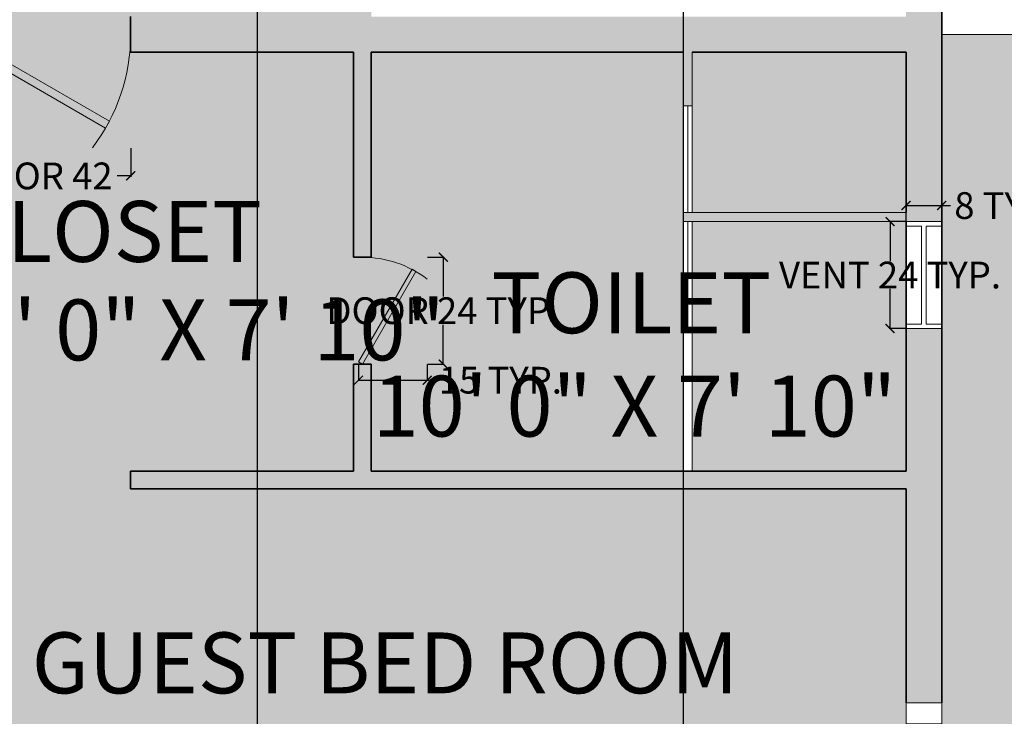
# Model space of a CAD drawing. Units: inches. Extents: x 1704 to 6393, y -157 to 1172.
# Tile 37 of 122: x 2398 to 2619, y 215 to 372. Entities that reach past the tile are written whole.
import ezdxf

# ---------------------------------------------------------------- set-up
doc = ezdxf.new("R2010")
doc.units = ezdxf.units.IN
doc.header["$MEASUREMENT"] = 0
for name, color, linetype, lineweight in [('A-ANNO-DIMS', 7, 'Continuous', 13), ('A-AREA-IDEN', 7, 'Continuous', 18), ('A-WALL-PATT', 7, 'Continuous', 13), ('DOORS', 160, 'Continuous', 18), ('GLASS PANEL FASADE', 4, 'Continuous', 18), ('L-HRDS', 8, 'Continuous', 18), ('L-PVMT-PATT', 8, 'Continuous', 13), ('WALLS', 7, 'Continuous', 35), ('WINDOWS', 2, 'Continuous', 18)]:
    doc.layers.add(name, color=color, linetype=linetype, lineweight=lineweight)
doc.layers.add('A-FLOR-PATT', color=7, linetype='Continuous', lineweight=13, true_color=0xf2f2f2)
doc.layers.add('L-HRDS-PATT', color=9, linetype='Continuous', lineweight=13, true_color=0xc5c1ba)
doc.styles.get("Standard").update_dxf_attribs({"font": 'arial.ttf'})
doc.dimstyles.get("Standard").update_dxf_attribs({"dimtxt": 6, "dimasz": 2, "dimexe": 0.18, "dimexo": 0.0625, "dimgap": 0.09, "dimtad": 0, "dimtih": 1, "dimtoh": 1, "dimdec": 1, "dimzin": 0, "dimdsep": 46, "dimlunit": 3, "dimtxsty": 'Standard', "dimblk": 'ARCHTICK', "dimcen": 0.09, "dimadec": 0, "dimazin": 0, "dimtfac": 1, "dimtdec": 1, "dimtofl": 0, "dimtmove": 0, "dimatfit": 3, "dimfxl": 1, "dimtolj": 1, "dimtzin": 0, "dimarcsym": 0})

# ---------------------------------------------------------------- blocks, each defined once
blk = doc.blocks.new('Door - Left Hung 36 in.')
blk.add_lwpolyline([(0.75, -1.3), (0, 0), (31.18, 18), (31.93, 16.7)], close=True)
blk.add_arc((0, 0), 36, 0, 37.3101)
blk = doc.blocks.new('WIN-SLIDER-72')
for p, q in [((0, 72), (0, 0)), ((0, 72), (8, 72)), ((8, 66.25), (8, 72)), ((0, 67.23), (8, 67.23)), ((1.17, 36), (1.17, 64.3)), ((8, 7.7), (8, 64.3)), ((3.12, 37.95), (3.12, 62.35)), ((4.1, 37.95), (4.1, 62.35)), ((5.07, 37.95), (5.07, 62.35)), ((2.14, 37.95), (2.14, 42.14)), ((5.07, 36), (5.07, 7.7)), ((1.17, 9.65), (1.17, 34.05)), ((2.14, 9.65), (2.14, 34.05)), ((3.12, 9.65), (3.12, 34.05)), ((4.1, 34.05), (4.1, 29.86)), ((0, 4.77), (8, 4.77)), ((8, 5.75), (8, 0)), ((0, 0), (8, 0))]:
    blk.add_line(p, q)
for points in [[(8, 64.3), (8, 66.25), (0, 66.25), (0, 64.3)], [(5.07, 62.35), (5.07, 64.3), (3.12, 64.3), (3.12, 62.35)], [(2.14, 42.65), (1.85, 42.14), (2.44, 42.14)], [(5.07, 36), (5.07, 37.95), (3.12, 37.95), (3.12, 36)], [(3.12, 34.05), (3.12, 36), (1.17, 36), (1.17, 34.05)], [(4.1, 29.35), (3.8, 29.86), (4.39, 29.86)], [(3.12, 7.7), (3.12, 9.65), (1.17, 9.65), (1.17, 7.7)], [(8, 7.7), (8, 5.75), (0, 5.75), (0, 7.7)]]:
    blk.add_lwpolyline(points, close=True)
blk = doc.blocks.new('WIN-VENT-24')
for p, q in [((0, 0), (0, 24)), ((0, 24), (8, 24)), ((0, 23), (3.5, 23)), ((3.5, 23), (3.5, 1)), ((4.5, 23), (8, 23)), ((4.5, 23), (4.5, 1)), ((8, 24), (8, 0)), ((3.5, 1), (0, 1)), ((8, 1), (4.5, 1)), ((8, 0), (0, 0))]:
    blk.add_line(p, q)
blk = doc.blocks.new('_ArchTick')
at = {"color": 0, "linetype": 'ByBlock', "const_width": 0.15}
blk.add_lwpolyline([(-0.5, -0.5), (0.5, 0.5)], dxfattribs=at)
blk = doc.blocks.new('*D30')
at = {"layer": 'A-ANNO-DIMS', "color": 0, "lineweight": -2, "transparency": 16777216}
for p, q in [((2381.35, 342.69), (2381.35, 336.28)), ((2423.35, 342.69), (2423.35, 336.28)), ((2381.35, 336.46), (2384.4, 336.46)), ((2423.35, 336.46), (2420.29, 336.46))]:
    blk.add_line(p, q, dxfattribs=at)
at = {"layer": 'Defpoints', "color": 0, "lineweight": -3, "transparency": 16777216}
for p in [(2381.35, 342.76), (2423.35, 342.76), (2423.35, 336.46)]:
    blk.add_point(p, dxfattribs=at)
at = {"layer": 'A-ANNO-DIMS', "color": 0, "lineweight": -2, "transparency": 16777216, "xscale": 2, "yscale": 2, "zscale": 2, "rotation": 180}
blk.add_blockref('_ArchTick', (2381.35, 336.46), dxfattribs=at)
at = {"layer": 'A-ANNO-DIMS', "color": 0, "lineweight": -2, "transparency": 16777216, "xscale": 2, "yscale": 2, "zscale": 2}
blk.add_blockref('_ArchTick', (2423.35, 336.46), dxfattribs=at)
at = {"layer": 'A-ANNO-DIMS', "color": 0, "transparency": 16777216, "insert": (2402.35, 336.46), "char_height": 6, "attachment_point": 5}
blk.add_mtext('\\A1;DOOR 42', dxfattribs=at)
blk = doc.blocks.new('*D32')
at = {"layer": 'A-ANNO-DIMS', "color": 0, "lineweight": -2, "transparency": 16777216}
for p, q in [((2489.96, 318.21), (2493.68, 318.21)), ((2493.5, 318.21), (2493.5, 309.41)), ((2493.5, 294.21), (2493.5, 303.02)), ((2489.96, 294.21), (2493.68, 294.21))]:
    blk.add_line(p, q, dxfattribs=at)
at = {"layer": 'Defpoints', "color": 0, "lineweight": -3, "transparency": 16777216}
for p in [(2489.9, 318.21), (2493.5, 318.21), (2489.9, 294.21)]:
    blk.add_point(p, dxfattribs=at)
at = {"layer": 'A-ANNO-DIMS', "color": 0, "lineweight": -2, "transparency": 16777216, "xscale": 2, "yscale": 2, "zscale": 2}
for p, rotation in [((2493.5, 318.21), 90), ((2493.5, 294.21), 270)]:
    blk.add_blockref('_ArchTick', p, dxfattribs=dict(at, rotation=rotation))
at = {"layer": 'A-ANNO-DIMS', "color": 0, "transparency": 16777216, "insert": (2493.5, 306.21), "char_height": 6, "attachment_point": 5}
blk.add_mtext('\\A1;DOOR 24 TYP.', dxfattribs=at)
blk = doc.blocks.new('*D33')
at = {"layer": 'A-ANNO-DIMS', "color": 0, "lineweight": -2, "transparency": 16777216}
for p, q in [((2474.48, 294.15), (2474.48, 290.43)), ((2489.9, 294.15), (2489.9, 290.43)), ((2474.48, 290.61), (2489.9, 290.61)), ((2489.9, 290.61), (2491.9, 290.61))]:
    blk.add_line(p, q, dxfattribs=at)
at = {"layer": 'Defpoints', "color": 0, "lineweight": -3, "transparency": 16777216}
for p in [(2474.48, 294.21), (2489.9, 294.21), (2489.9, 290.61)]:
    blk.add_point(p, dxfattribs=at)
at = {"layer": 'A-ANNO-DIMS', "color": 0, "lineweight": -2, "transparency": 16777216, "xscale": 2, "yscale": 2, "zscale": 2, "rotation": 180}
blk.add_blockref('_ArchTick', (2474.48, 290.61), dxfattribs=at)
at = {"layer": 'A-ANNO-DIMS', "color": 0, "lineweight": -2, "transparency": 16777216, "xscale": 2, "yscale": 2, "zscale": 2}
blk.add_blockref('_ArchTick', (2489.9, 290.61), dxfattribs=at)
at = {"layer": 'A-ANNO-DIMS', "color": 0, "transparency": 16777216, "insert": (2506.31, 290.61), "char_height": 6, "attachment_point": 5}
blk.add_mtext('\\A1;15 TYP.', dxfattribs=at)
blk = doc.blocks.new('*D42')
at = {"layer": 'A-ANNO-DIMS', "color": 0, "lineweight": -2, "transparency": 16777216}
for p, q in [((2597.29, 326.21), (2593.57, 326.21)), ((2593.75, 326.21), (2593.75, 317.32)), ((2593.75, 302.21), (2593.75, 311.11)), ((2597.29, 302.21), (2593.57, 302.21))]:
    blk.add_line(p, q, dxfattribs=at)
at = {"layer": 'Defpoints', "color": 0, "lineweight": -3, "transparency": 16777216}
for p in [(2593.75, 326.21), (2597.35, 326.21), (2597.35, 302.21)]:
    blk.add_point(p, dxfattribs=at)
at = {"layer": 'A-ANNO-DIMS', "color": 0, "lineweight": -2, "transparency": 16777216, "xscale": 2, "yscale": 2, "zscale": 2}
for p, rotation in [((2593.75, 326.21), 90), ((2593.75, 302.21), 270)]:
    blk.add_blockref('_ArchTick', p, dxfattribs=dict(at, rotation=rotation))
at = {"layer": 'A-ANNO-DIMS', "color": 0, "transparency": 16777216, "insert": (2593.75, 314.21), "char_height": 6, "attachment_point": 5}
blk.add_mtext('\\A1;VENT 24 TYP.', dxfattribs=at)
blk = doc.blocks.new('*D43')
at = {"layer": 'A-ANNO-DIMS', "color": 0, "lineweight": -2, "transparency": 16777216}
for p, q in [((2597.35, 326.28), (2597.35, 329.99)), ((2597.35, 329.81), (2605.35, 329.81)), ((2605.35, 326.28), (2605.35, 329.99)), ((2605.35, 329.81), (2607.35, 329.81))]:
    blk.add_line(p, q, dxfattribs=at)
at = {"layer": 'Defpoints', "color": 0, "lineweight": -3, "transparency": 16777216}
for p in [(2605.35, 329.81), (2597.35, 326.21), (2605.35, 326.21)]:
    blk.add_point(p, dxfattribs=at)
at = {"layer": 'A-ANNO-DIMS', "color": 0, "lineweight": -2, "transparency": 16777216, "xscale": 2, "yscale": 2, "zscale": 2, "rotation": 180}
blk.add_blockref('_ArchTick', (2597.35, 329.81), dxfattribs=at)
at = {"layer": 'A-ANNO-DIMS', "color": 0, "lineweight": -2, "transparency": 16777216, "xscale": 2, "yscale": 2, "zscale": 2}
blk.add_blockref('_ArchTick', (2605.35, 329.81), dxfattribs=at)
at = {"layer": 'A-ANNO-DIMS', "color": 0, "transparency": 16777216, "insert": (2619.71, 329.81), "char_height": 6, "attachment_point": 5}
blk.add_mtext('\\A1;8 TYP.', dxfattribs=at)
blk = doc.blocks.new('*D93')
at = {"layer": 'A-ANNO-DIMS', "color": 0, "lineweight": -2, "transparency": 16777216}
for p, q in [((2605.29, 895.21), (1829.7, 895.21)), ((1829.88, 895.21), (1829.88, 495.87)), ((1829.88, 90.21), (1829.88, 489.56)), ((2605.29, 90.21), (1829.7, 90.21))]:
    blk.add_line(p, q, dxfattribs=at)
at = {"layer": 'Defpoints', "color": 0, "lineweight": -3, "transparency": 16777216}
for p in [(2605.35, 895.21), (1829.88, 90.21), (2605.35, 90.21)]:
    blk.add_point(p, dxfattribs=at)
at = {"layer": 'A-ANNO-DIMS', "color": 0, "lineweight": -2, "transparency": 16777216, "xscale": 2, "yscale": 2, "zscale": 2}
for p, rotation in [((1829.88, 895.21), 90), ((1829.88, 90.21), 270)]:
    blk.add_blockref('_ArchTick', p, dxfattribs=dict(at, rotation=rotation))
at = {"layer": 'A-ANNO-DIMS', "color": 0, "transparency": 16777216, "insert": (1829.88, 492.71), "char_height": 6, "attachment_point": 5}
blk.add_mtext('\\A1;805', dxfattribs=at)
blk = doc.blocks.new('*D105')
at = {"layer": 'A-ANNO-DIMS', "color": 0, "lineweight": -2, "transparency": 16777216}
for p, q in [((2451.74, 615.15), (2451.74, -64.97)), ((2547.35, 615.15), (2547.35, -64.97)), ((2451.74, -64.79), (2489.91, -64.79)), ((2547.35, -64.79), (2509.18, -64.79))]:
    blk.add_line(p, q, dxfattribs=at)
at = {"layer": 'Defpoints', "color": 0, "lineweight": -3, "transparency": 16777216}
for p in [(2451.74, 615.21), (2547.35, 615.21), (2547.35, -64.79)]:
    blk.add_point(p, dxfattribs=at)
at = {"layer": 'A-ANNO-DIMS', "color": 0, "lineweight": -2, "transparency": 16777216, "xscale": 2, "yscale": 2, "zscale": 2, "rotation": 180}
blk.add_blockref('_ArchTick', (2451.74, -64.79), dxfattribs=at)
at = {"layer": 'A-ANNO-DIMS', "color": 0, "lineweight": -2, "transparency": 16777216, "xscale": 2, "yscale": 2, "zscale": 2}
blk.add_blockref('_ArchTick', (2547.35, -64.79), dxfattribs=at)
at = {"layer": 'A-ANNO-DIMS', "color": 0, "transparency": 16777216, "insert": (2499.54, -64.79), "char_height": 6, "attachment_point": 5}
blk.add_mtext('\\A1;95.61', dxfattribs=at)

msp = doc.modelspace()

# ---------------------------------------------------------------- hatches: boundary and pattern name
at = {"layer": 'A-FLOR-PATT', "transparency": 33554528}
h = msp.add_hatch(color=256, dxfattribs=at)
h.dxf.hatch_style = 1
h.paths.add_polyline_path([(2325.349, 863.213), (2325.349, 887.213), (2263.349, 887.213), (2167.349, 887.213), (2081.349, 887.213), (2081.349, 719.213), (2277.349, 719.213), (2277.349, 711.213), (2277.349, 372.213), (2349.349, 372.213), (2381.349, 372.213), (2381.349, 364.213), (2353.349, 364.213), (2353.349, 270.213), (2381.349, 270.213), (2381.349, 266.213), (2357.349, 266.213), (2357.349, 98.213), (2381.349, 98.213), (2385.181, 98.213), (2386.482, 98.213), (2424.215, 98.213), (2425.516, 98.213), (2429.349, 98.213), (2597.349, 98.213), (2597.349, 146.213), (2597.349, 218.213), (2597.349, 266.213), (2423.349, 266.213), (2423.349, 270.213), (2473.349, 270.213), (2473.349, 294.213), (2477.349, 294.213), (2477.349, 270.213), (2547.349, 270.213), (2547.349, 364.213), (2477.349, 364.213), (2477.349, 318.213), (2473.349, 318.213), (2473.349, 364.213), (2423.349, 364.213), (2423.349, 372.213), (2469.349, 372.213), (2469.349, 459.213), (2469.349, 538.213), (2350.349, 538.213), (2350.349, 565.713), (2358.349, 565.713), (2358.349, 545.213), (2420.349, 545.213), (2420.349, 610.213), (2358.349, 610.213), (2358.349, 589.713), (2350.349, 589.713), (2350.349, 615.213), (2425.349, 615.213), (2425.349, 607.213), (2425.349, 546.213), (2469.349, 546.213), (2514.349, 546.213), (2514.349, 607.213), (2449.349, 607.213), (2449.349, 615.213), (2451.738, 615.213), (2451.738, 659.213), (2427.738, 659.213), (2427.738, 665.213), (2367.738, 665.213), (2367.738, 667.213), (2367.738, 711.213), (2325.349, 711.213), (2325.349, 719.213), (2325.349, 755.213), (2325.349, 763.213)])
h.paths.add_polyline_path([(2233.858, 822.533, -0.187247), (2233.858, 809.14), (2231.697, 808.804, 0.0848928), (2233.131, 814.486), (2230.424, 814.486, -0.1042581), (2228.553, 808.313), (2217.751, 807.156, -0.2222222), (2217.751, 824.517), (2228.553, 823.359, -0.1042581), (2230.424, 817.186), (2233.131, 817.186, 0.0848928), (2231.697, 822.868)], flags=16)
h.paths.add_polyline_path([(2213.621, 833.197), (2213.621, 798.475), (2156.048, 798.475), (2156.048, 833.197)], flags=16)
h.paths.add_polyline_path([(2203.932, 848.099), (2205.089, 837.296, -0.2222222), (2187.728, 837.296), (2188.885, 848.099, -0.1042581), (2195.058, 849.969), (2195.058, 852.676, 0.0848928), (2189.377, 851.242), (2189.712, 853.404, -0.187247), (2203.105, 853.404), (2203.44, 851.242, 0.0848928), (2197.759, 852.676), (2197.759, 849.969, -0.1042581)], flags=16)
h.paths.add_polyline_path([(2181.941, 837.296, -0.2222222), (2164.58, 837.296), (2165.737, 848.099, -0.1042581), (2171.91, 849.969), (2171.91, 852.676, 0.0848928), (2166.229, 851.242), (2166.564, 853.404, -0.187247), (2179.957, 853.404), (2180.292, 851.242, 0.0848928), (2174.611, 852.676), (2174.611, 849.969, -0.1042581), (2180.784, 848.099)], flags=16)
h.paths.add_polyline_path([(2205.089, 794.376), (2203.932, 783.574, -0.1042581), (2197.759, 781.703), (2197.759, 778.996, 0.0848928), (2203.44, 780.43), (2203.105, 778.269, -0.187247), (2189.712, 778.269), (2189.377, 780.43, 0.0848928), (2195.058, 778.996), (2195.058, 781.703, -0.1042581), (2188.885, 783.574), (2187.728, 794.376, -0.2222222)], flags=16)
h.paths.add_polyline_path([(2181.941, 794.376), (2180.784, 783.574, -0.1042581), (2174.611, 781.703), (2174.611, 778.996, 0.0848928), (2180.292, 780.43), (2179.957, 778.269, -0.187247), (2166.564, 778.269), (2166.229, 780.43, 0.0848928), (2171.91, 778.996), (2171.91, 781.703, -0.1042581), (2165.737, 783.574), (2164.58, 794.376, -0.2222222)], flags=16)
h.paths.add_polyline_path([(2151.918, 807.156), (2141.116, 808.313, -0.1042581), (2139.245, 814.486), (2136.539, 814.486, 0.0848928), (2137.972, 808.804), (2135.811, 809.14, -0.187247), (2135.811, 822.533), (2137.972, 822.868, 0.0848928), (2136.539, 817.186), (2139.245, 817.186, -0.1042581), (2141.116, 823.359), (2151.918, 824.517, -0.2222222)], flags=16)
h.paths.add_polyline_path([(2357.868, 363.41), (2358.814, 363.41, 0.7537605)], flags=16)
h.paths.add_polyline_path([(2372.241, 363.117), (2372.248, 363.117), (2372.248, 363.343), (2371.302, 363.343), (2371.302, 363.139, -1.3603913)], flags=16)
h.paths.add_polyline_path([(2371.309, 272.716), (2371.302, 272.716), (2371.302, 272.49), (2372.248, 272.49), (2372.248, 272.693, -1.3603913)], flags=16)
h.paths.add_polyline_path([(2357.875, 272.716), (2357.868, 272.716), (2357.868, 272.49), (2358.814, 272.49), (2358.814, 272.693, -1.3603913)], flags=16)
h.paths.add_polyline_path([(2353.769, 363.074), (2376.347, 363.074), (2376.347, 272.759), (2353.769, 272.759)], flags=16)
h.paths.add_polyline_path([(2354.772, 362.07), (2375.344, 362.07), (2375.344, 273.762), (2354.772, 273.762)], flags=0)
h.paths.add_polyline_path([(2357.868, 363.343), (2358.814, 363.343), (2358.814, 363.117), (2357.868, 363.117)], flags=16)
h.paths.add_polyline_path([(2359.288, 359.184), (2359.288, 360.063), (2370.828, 360.063), (2370.828, 359.184), (2374.332, 359.184), (2374.332, 358.464), (2372.835, 358.464), (2372.835, 357.541), (2374.332, 357.541), (2374.332, 356.82), (2372.835, 356.82), (2372.835, 355.898), (2374.332, 355.898), (2374.332, 355.177), (2372.835, 355.177), (2372.835, 354.254), (2374.332, 354.254), (2374.332, 353.534), (2372.835, 353.534), (2372.835, 352.611), (2374.332, 352.611), (2374.332, 351.89), (2372.835, 351.89), (2372.835, 350.968), (2374.332, 350.968), (2374.332, 350.247), (2372.835, 350.247), (2372.835, 349.324), (2374.332, 349.324), (2374.332, 348.604), (2372.835, 348.604), (2372.835, 347.681), (2374.332, 347.681), (2374.332, 346.96), (2372.835, 346.96), (2372.835, 346.038), (2374.332, 346.038), (2374.332, 345.317), (2372.835, 345.317), (2372.835, 344.395), (2374.332, 344.395), (2374.332, 343.674), (2372.835, 343.674), (2372.835, 342.751), (2374.332, 342.751), (2374.332, 342.03), (2372.835, 342.03), (2372.835, 341.108), (2374.332, 341.108), (2374.332, 340.387), (2372.835, 340.387), (2372.835, 339.465), (2374.332, 339.465), (2374.332, 338.744), (2372.835, 338.744), (2372.835, 337.821), (2374.332, 337.821), (2374.332, 337.1), (2372.835, 337.1), (2372.835, 336.178), (2374.332, 336.178), (2374.332, 335.457), (2372.835, 335.457), (2372.835, 334.535), (2374.332, 334.535), (2374.332, 333.814), (2372.835, 333.814), (2372.835, 332.891), (2374.332, 332.891), (2374.332, 332.171), (2372.835, 332.171), (2372.835, 331.248), (2374.332, 331.248), (2374.332, 330.527), (2372.835, 330.527), (2372.835, 329.605), (2374.332, 329.605), (2374.332, 328.884), (2372.835, 328.884), (2372.835, 327.961), (2374.332, 327.961), (2374.332, 327.241), (2372.835, 327.241), (2372.835, 326.318), (2374.332, 326.318), (2374.332, 325.597), (2372.835, 325.597), (2372.835, 324.675), (2374.332, 324.675), (2374.332, 323.954), (2372.835, 323.954), (2372.835, 323.031), (2374.332, 323.031), (2374.332, 322.311), (2372.835, 322.311), (2372.835, 321.388), (2374.332, 321.388), (2374.332, 320.667), (2372.835, 320.667), (2372.835, 319.745), (2374.332, 319.745), (2374.332, 319.024), (2372.835, 319.024), (2372.835, 318.102), (2374.332, 318.102), (2374.332, 317.381), (2372.835, 317.381), (2372.835, 316.458), (2374.332, 316.458), (2374.332, 315.737), (2372.835, 315.737), (2372.835, 314.815), (2374.332, 314.815), (2374.332, 314.094), (2372.835, 314.094), (2372.835, 313.172), (2374.332, 313.172), (2374.332, 312.451), (2372.835, 312.451), (2372.835, 311.528), (2374.332, 311.528), (2374.332, 310.807), (2372.835, 310.807), (2372.835, 309.885), (2374.332, 309.885), (2374.332, 309.164), (2372.835, 309.164), (2372.835, 308.242), (2374.332, 308.242), (2374.332, 307.521), (2372.835, 307.521), (2372.835, 306.598), (2374.332, 306.598), (2374.332, 305.878), (2372.835, 305.878), (2372.835, 304.955), (2374.332, 304.955), (2374.332, 304.234), (2372.835, 304.234), (2372.835, 303.312), (2374.332, 303.312), (2374.332, 302.591), (2372.835, 302.591), (2372.835, 301.668), (2374.332, 301.668), (2374.332, 300.948), (2372.835, 300.948), (2372.835, 300.025), (2374.332, 300.025), (2374.332, 299.304), (2372.835, 299.304), (2372.835, 298.382), (2374.332, 298.382), (2374.332, 297.661), (2372.835, 297.661), (2372.835, 296.738), (2374.332, 296.738), (2374.332, 296.018), (2372.835, 296.018), (2372.835, 295.095), (2374.332, 295.095), (2374.332, 294.374), (2372.835, 294.374), (2372.835, 293.452), (2374.332, 293.452), (2374.332, 292.731), (2372.835, 292.731), (2372.835, 291.809), (2374.332, 291.809), (2374.332, 291.088), (2372.835, 291.088), (2372.835, 290.165), (2374.332, 290.165), (2374.332, 289.444), (2372.835, 289.444), (2372.835, 288.522), (2374.332, 288.522), (2374.332, 287.801), (2372.835, 287.801), (2372.835, 286.879), (2374.332, 286.879), (2374.332, 286.158), (2372.835, 286.158), (2372.835, 285.235), (2374.332, 285.235), (2374.332, 284.514), (2372.835, 284.514), (2372.835, 283.592), (2374.332, 283.592), (2374.332, 282.871), (2372.835, 282.871), (2372.835, 281.949), (2374.332, 281.949), (2374.332, 281.228), (2372.835, 281.228), (2372.835, 280.305), (2374.332, 280.305), (2374.332, 279.585), (2372.835, 279.585), (2372.835, 278.662), (2374.332, 278.662), (2374.332, 277.941), (2372.835, 277.941), (2372.835, 277.019), (2374.332, 277.019), (2374.332, 276.298), (2370.828, 276.298), (2370.828, 275.769), (2359.288, 275.769), (2359.288, 276.298), (2355.784, 276.298), (2355.784, 277.019), (2357.281, 277.019), (2357.281, 277.941), (2355.784, 277.941), (2355.784, 278.662), (2357.281, 278.662), (2357.281, 279.585), (2355.784, 279.585), (2355.784, 280.305), (2357.281, 280.305), (2357.281, 281.228), (2355.784, 281.228), (2355.784, 281.949), (2357.281, 281.949), (2357.281, 282.871), (2355.784, 282.871), (2355.784, 283.592), (2357.281, 283.592), (2357.281, 284.514), (2355.784, 284.514), (2355.784, 285.235), (2357.281, 285.235), (2357.281, 286.158), (2355.784, 286.158), (2355.784, 286.879), (2357.281, 286.879), (2357.281, 287.801), (2355.784, 287.801), (2355.784, 288.522), (2357.281, 288.522), (2357.281, 289.444), (2355.784, 289.444), (2355.784, 290.165), (2357.281, 290.165), (2357.281, 291.088), (2355.784, 291.088), (2355.784, 291.809), (2357.281, 291.809), (2357.281, 292.731), (2355.784, 292.731), (2355.784, 293.452), (2357.281, 293.452), (2357.281, 294.374), (2355.784, 294.374), (2355.784, 295.095), (2357.281, 295.095), (2357.281, 296.018), (2355.784, 296.018), (2355.784, 296.738), (2357.281, 296.738), (2357.281, 297.661), (2355.784, 297.661), (2355.784, 298.382), (2357.281, 298.382), (2357.281, 299.304), (2355.784, 299.304), (2355.784, 300.025), (2357.281, 300.025), (2357.281, 300.948), (2355.784, 300.948), (2355.784, 301.668), (2357.281, 301.668), (2357.281, 302.591), (2355.784, 302.591), (2355.784, 303.312), (2357.281, 303.312), (2357.281, 304.234), (2355.784, 304.234), (2355.784, 304.955), (2357.281, 304.955), (2357.281, 305.878), (2355.784, 305.878), (2355.784, 306.598), (2357.281, 306.598), (2357.281, 307.521), (2355.784, 307.521), (2355.784, 308.242), (2357.281, 308.242), (2357.281, 309.164), (2355.784, 309.164), (2355.784, 309.885), (2357.281, 309.885), (2357.281, 310.807), (2355.784, 310.807), (2355.784, 311.528), (2357.281, 311.528), (2357.281, 312.451), (2355.784, 312.451), (2355.784, 313.172), (2357.281, 313.172), (2357.281, 314.094), (2355.784, 314.094), (2355.784, 314.815), (2357.281, 314.815), (2357.281, 315.737), (2355.784, 315.737), (2355.784, 316.458), (2357.281, 316.458), (2357.281, 317.381), (2355.784, 317.381), (2355.784, 318.102), (2357.281, 318.102), (2357.281, 319.024), (2355.784, 319.024), (2355.784, 319.745), (2357.281, 319.745), (2357.281, 320.667), (2355.784, 320.667), (2355.784, 321.388), (2357.281, 321.388), (2357.281, 322.311), (2355.784, 322.311), (2355.784, 323.031), (2357.281, 323.031), (2357.281, 323.954), (2355.784, 323.954), (2355.784, 324.675), (2357.281, 324.675), (2357.281, 325.597), (2355.784, 325.597), (2355.784, 326.318), (2357.281, 326.318), (2357.281, 327.241), (2355.784, 327.241), (2355.784, 327.961), (2357.281, 327.961), (2357.281, 328.884), (2355.784, 328.884), (2355.784, 329.605), (2357.281, 329.605), (2357.281, 330.527), (2355.784, 330.527), (2355.784, 331.248), (2357.281, 331.248), (2357.281, 332.171), (2355.784, 332.171), (2355.784, 332.891), (2357.281, 332.891), (2357.281, 333.814), (2355.784, 333.814), (2355.784, 334.535), (2357.281, 334.535), (2357.281, 335.457), (2355.784, 335.457), (2355.784, 336.178), (2357.281, 336.178), (2357.281, 337.1), (2355.784, 337.1), (2355.784, 337.821), (2357.281, 337.821), (2357.281, 338.744), (2355.784, 338.744), (2355.784, 339.465), (2357.281, 339.465), (2357.281, 340.387), (2355.784, 340.387), (2355.784, 341.108), (2357.281, 341.108), (2357.281, 342.03), (2355.784, 342.03), (2355.784, 342.751), (2357.281, 342.751), (2357.281, 343.674), (2355.784, 343.674), (2355.784, 344.395), (2357.281, 344.395), (2357.281, 345.317), (2355.784, 345.317), (2355.784, 346.038), (2357.281, 346.038), (2357.281, 346.96), (2355.784, 346.96), (2355.784, 347.681), (2357.281, 347.681), (2357.281, 348.604), (2355.784, 348.604), (2355.784, 349.324), (2357.281, 349.324), (2357.281, 350.247), (2355.784, 350.247), (2355.784, 350.968), (2357.281, 350.968), (2357.281, 351.89), (2355.784, 351.89), (2355.784, 352.611), (2357.281, 352.611), (2357.281, 353.534), (2355.784, 353.534), (2355.784, 354.254), (2357.281, 354.254), (2357.281, 355.177), (2355.784, 355.177), (2355.784, 355.898), (2357.281, 355.898), (2357.281, 356.82), (2355.784, 356.82), (2355.784, 357.541), (2357.281, 357.541), (2357.281, 358.464), (2355.784, 358.464), (2355.784, 359.184)], flags=0)
h = msp.add_hatch(color=256, dxfattribs=at)
h.dxf.hatch_style = 1
h.paths.add_polyline_path([(2597.349, 326.213), (2549.349, 326.213), (2549.349, 270.213), (2597.349, 270.213)])
h.paths.add_polyline_path([(2597.349, 364.213), (2549.349, 364.213), (2549.349, 328.213), (2597.349, 328.213)])
at = {"layer": 'A-WALL-PATT', "transparency": 33554643}
h = msp.add_hatch(color=256, dxfattribs=at)
h.dxf.hatch_style = 1
h.paths.add_polyline_path([(2167.349, 895.213), (2073.349, 895.213), (2073.349, 887.213), (2081.349, 887.213), (2167.349, 887.213)])
h.paths.add_polyline_path([(2465.349, 895.213), (2273.349, 895.213), (2273.349, 903.213), (2263.349, 903.213), (2263.349, 895.213), (2263.349, 887.213), (2325.349, 887.213), (2325.349, 863.213), (2333.349, 863.213), (2333.349, 887.213), (2465.349, 887.213)])
h.paths.add_polyline_path([(2533.349, 895.213), (2513.349, 895.213), (2513.349, 887.213), (2513.349, 861.213), (2517.349, 861.213), (2517.349, 887.213), (2533.349, 887.213)])
h.paths.add_polyline_path([(2605.349, 895.213), (2581.349, 895.213), (2581.349, 887.213), (2597.349, 887.213), (2597.349, 854.213), (2605.349, 854.213)])
h.paths.add_polyline_path([(2605.349, 752.213), (2629.349, 752.213), (2629.349, 716.213), (2605.349, 716.213), (2605.349, 712.213), (2719.349, 712.213), (2719.349, 716.213), (2631.349, 716.213), (2631.349, 754.213), (2605.349, 754.213), (2605.349, 794.213), (2597.349, 794.213), (2597.349, 787.213), (2517.349, 787.213), (2517.349, 813.213), (2513.349, 813.213), (2513.349, 783.213), (2517.349, 783.213), (2597.349, 783.213), (2597.349, 719.213), (2517.349, 719.213), (2517.349, 753.213), (2513.349, 753.213), (2513.349, 719.213), (2365.349, 719.213), (2365.349, 763.213), (2325.349, 763.213), (2325.349, 755.213), (2357.349, 755.213), (2357.349, 719.213), (2325.349, 719.213), (2325.349, 711.213), (2547.349, 711.213), (2547.349, 615.213), (2449.349, 615.213), (2449.349, 607.213), (2514.349, 607.213), (2514.349, 546.213), (2439.349, 546.213), (2425.349, 546.213), (2425.349, 607.213), (2425.349, 615.213), (2350.349, 615.213), (2350.349, 589.713), (2358.349, 589.713), (2358.349, 610.213), (2420.349, 610.213), (2420.349, 545.213), (2358.349, 545.213), (2358.349, 565.713), (2350.349, 565.713), (2350.349, 538.213), (2469.349, 538.213), (2469.349, 459.213), (2469.349, 372.213), (2423.349, 372.213), (2423.349, 364.213), (2473.349, 364.213), (2473.349, 318.213), (2477.349, 318.213), (2477.349, 364.213), (2547.349, 364.213), (2547.349, 352.213), (2549.349, 352.213), (2549.349, 364.213), (2597.349, 364.213), (2597.349, 328.213), (2549.349, 328.213), (2547.349, 328.213), (2547.349, 326.213), (2549.349, 326.213), (2597.349, 326.213), (2605.349, 326.213), (2605.349, 377.057), (2597.349, 377.057), (2597.349, 372.213), (2477.349, 372.213), (2477.349, 451.213), (2597.349, 451.213), (2605.349, 451.213), (2605.349, 459.213), (2597.349, 459.213), (2477.349, 459.213), (2477.349, 538.213), (2597.349, 538.213), (2597.349, 495.213), (2605.349, 495.213), (2605.349, 512.213), (2631.349, 512.213), (2631.349, 568.213), (2605.349, 568.213), (2605.349, 577.213), (2597.349, 577.213), (2597.349, 542.213), (2518.349, 542.213), (2518.349, 607.213), (2532.349, 607.213), (2605.349, 607.213), (2605.349, 615.213), (2597.349, 615.213), (2551.349, 615.213), (2551.349, 711.213), (2597.349, 711.213), (2597.349, 645.213), (2605.349, 645.213), (2605.349, 712.213), (2605.349, 716.213)])
h.paths.add_polyline_path([(2605.349, 566.213), (2629.349, 566.213), (2629.349, 514.213), (2605.349, 514.213)], flags=16)
h.paths.add_polyline_path([(2381.349, 372.213), (2349.349, 372.213), (2349.349, 202.213), (2337.349, 202.213), (2337.349, 194.213), (2349.349, 194.213), (2349.349, 90.213), (2349.349, 72.213), (2357.349, 72.213), (2357.349, 90.213), (2381.349, 90.213), (2381.349, 98.213), (2357.349, 98.213), (2357.349, 266.213), (2381.349, 266.213), (2381.349, 270.213), (2353.349, 270.213), (2353.349, 364.213), (2381.349, 364.213)])
h.paths.add_polyline_path([(2605.349, 302.213), (2597.349, 302.213), (2597.349, 270.213), (2477.349, 270.213), (2477.349, 294.213), (2473.349, 294.213), (2473.349, 270.213), (2423.349, 270.213), (2423.349, 266.213), (2597.349, 266.213), (2597.349, 218.213), (2605.349, 218.213)])
h.paths.add_polyline_path([(2605.349, 146.213), (2597.349, 146.213), (2597.349, 98.213), (2429.349, 98.213), (2429.349, 90.213), (2597.349, 90.213), (2597.349, 72.213), (2605.349, 72.213), (2605.349, 90.213)])
h.paths.add_polyline_path([(2225.349, 202.213), (2049.349, 202.213), (2049.349, 194.213), (2225.349, 194.213)])
h.paths.add_polyline_path([(2289.349, 202.213), (2277.349, 202.213), (2273.349, 202.213), (2269.516, 202.213), (2269.516, 194.213), (2273.349, 194.213), (2277.349, 194.213), (2289.349, 194.213)])
h.paths.add_polyline_path([(2273.349, 372.213), (2029.19, 372.213), (2029.19, 364.213), (2273.349, 364.213)])
h.paths.add_polyline_path([(2277.349, 545.213), (2213.349, 545.213), (2213.349, 573.213), (2205.349, 573.213), (2177.349, 573.213), (2177.349, 545.213), (2073.349, 545.213), (2073.349, 538.213), (2081.349, 538.213), (2277.349, 538.213)])
h.paths.add_polyline_path([(2181.349, 545.213), (2181.349, 569.213), (2205.349, 569.213), (2205.349, 545.213)], flags=16)
h.paths.add_polyline_path([(2277.349, 719.213), (2081.349, 719.213), (2073.349, 719.213), (2073.349, 711.213), (2154.575, 711.213), (2205.349, 711.213), (2205.349, 687.213), (2205.349, 629.213), (2213.349, 629.213), (2273.349, 629.213), (2273.349, 631.213), (2207.349, 631.213), (2207.349, 707.213), (2231.349, 707.213), (2231.349, 709.213), (2207.349, 709.213), (2207.349, 711.213), (2277.349, 711.213)])
at = {"layer": 'L-HRDS-PATT', "transparency": 33554539}
h = msp.add_hatch(color=256, dxfattribs=at)
h.dxf.hatch_style = 1
h.paths.add_polyline_path([(2651.217, 368.213), (2605.349, 368.213), (2605.349, 218.213), (2605.349, 212.464), (2605.349, 210.513), (2605.349, 153.913), (2605.349, 151.962), (2605.349, 146.213), (2605.349, 90.213), (2605.349, 72.213), (2601.349, 72.213), (2600.88, 50.634), (2719.349, 50.634), (2719.349, 72.213), (2711.349, 72.213), (2663.217, 72.213), (2651.217, 72.213)])
h.paths.add_polyline_path([(2711.349, 48.634), (2600.88, 48.634), (2576.88, 48.634), (2576.88, 17.658), (2711.349, 17.658)])
h.paths.add_polyline_path([(2601.349, 72.213), (2597.349, 72.213), (2597.349, 90.213), (2429.349, 90.213), (2425.516, 90.213), (2424.215, 90.213), (2386.482, 90.213), (2385.181, 90.213), (2381.349, 90.213), (2357.349, 90.213), (2357.349, 72.213), (2349.349, 72.213), (2349.349, 90.213), (2349.349, 134.213), (2277.349, 134.213), (2277.349, 50.634), (2566.88, 50.634), (2600.88, 50.634)])
h.paths.add_polyline_path([(2349.349, 146.213), (2277.349, 146.213), (2277.349, 134.213), (2349.349, 134.213)])
h.paths.add_polyline_path([(2349.349, 158.213), (2277.349, 158.213), (2277.349, 146.213), (2349.349, 146.213)])
h.paths.add_polyline_path([(2349.349, 170.213), (2277.349, 170.213), (2277.349, 158.213), (2349.349, 158.213)])
h.paths.add_polyline_path([(2349.349, 194.213), (2337.349, 194.213), (2337.349, 202.213), (2349.349, 202.213), (2349.349, 364.213), (2277.349, 364.213), (2277.349, 202.213), (2289.349, 202.213), (2289.349, 194.213), (2277.349, 194.213), (2277.349, 170.213), (2349.349, 170.213)])
at = {"layer": 'L-PVMT-PATT', "transparency": 33554643}
h = msp.add_hatch(dxfattribs=at)
h.set_pattern_fill('GRAVEL', color=256, scale=2.4)
h.set_pattern_definition([(228.0127875, (1.728, 2.4), (-19.2, -21.6), [0.3228864, -31.9658113]), (184.9697407, (1.512, 2.16), (28.8, 2.4), [0.5540832, -54.8542194]), (132.510447, (0.96, 2.112), (24, -26.4), [0.3906912, -38.6784782]), (267.273689, (0.024, 1.512), (2.4, 48), [0.5045712, -49.9525393]), (292.833654, (0, 1.008), (-12, 28.8), [0.494772, -48.9824955]), (357.273689, (0.192, 0.552), (-48, 2.4), [0.5045712, -49.9525393]), (37.6942405, (0.696, 0.528), (-31.2, -24), [0.6672696, -66.0596365]), (72.2553284, (1.224, 0.936), (16.8, 52.8), [0.6299712, -62.3671716]), (121.4295656, (1.416, 1.536), (-19.2, 31.2), [0.50628, -50.1217755]), (175.236358, (1.152, 1.968), (26.4, -2.4), [0.5779968, -28.3218302]), (222.3974378, (0.576, 2.016), (-28.8, -26.4), [0.7474752, -74.0001]), (138.814075, (2.4, 1.488), (-16.8, 14.4), [0.2551224, -25.2572276]), (171.4692344, (2.208, 1.656), (31.2, -4.8), [0.4853688, -48.0516274]), (225, (1.728, 1.728), (-3e-16, -2.4), [0.3394104, -3.0547021]), (203.19859, (1.56, 2.016), (12, 4.8), [0.1827792, -18.0950763]), (291.80141, (1.392, 1.944), (-2.4, 7.2), [0.2584872, -12.6659083]), (30.963757, (1.488, 1.704), (7.2, 4.8), [0.4198296, -13.574455]), (161.56505, (1.848, 1.92), (4.8, -2.4), [0.3035784, -7.285888]), (16.3895403, (0, 1.944), (24, 7.2), [0.42528, -42.1028284]), (70.346176, (0.408, 2.064), (-9.6, -26.4), [0.3567864, -35.3217786]), (293.19859, (1.848, 2.4), (-4.8, 12), [0.365556, -17.9122995]), (343.6104597, (1.992, 2.064), (-24, 7.2), [0.42528, -42.1028284]), (339.443955, (0, 0.456), (-12, 4.8), [0.410112, -20.095497]), (294.7751406, (0.384, 0.312), (-12, 26.4), [0.3436272, -34.0191434]), (66.80141, (1.872, 0), (4.8, 12), [0.365556, -17.9122995]), (17.3540246, (2.016, 0.336), (-31.2, -9.6), [0.4023144, -39.8290167]), (69.443955, (0.696, 0), (-4.8, -12), [0.205056, -20.300553]), (101.309932, (1.728, 0), (-2.4, 9.6), [0.122376, -12.1152708]), (165.963757, (1.704, 0.12), (7.2, -2.4), [0.494772, -9.4006815]), (186.009006, (1.224, 0.24), (24, 2.4), [0.45852, -45.3934156]), (303.690068, (1.488, 1.488), (-2.4, 4.8), [0.3461328, -8.3071903]), (353.1572266, (1.68, 1.2), (40.8, -4.8), [0.6043056, -59.8261503]), (60.945396, (2.28, 1.128), (-9.6, -16.8), [0.2470944, -24.462418]), (90, (2.4, 1.344), (-2.4, 2.4), [0.144, -2.256]), (120.256437, (1.176, 0.312), (9.6, -16.8), [0.3334176, -33.008448]), (48.0127875, (1.008, 0.6), (19.2, 21.6), [0.6457728, -31.642925]), (0, (1.44, 1.08), (2.4, 2.4), [0.624, -1.776]), (325.3048465, (2.064, 1.08), (24, -16.8), [0.3794736, -37.5678583]), (254.054604, (2.376, 0.864), (-2.4, -9.6), [0.3494448, -17.122819]), (207.6459754, (2.28, 0.528), (-45.6, -24), [0.568956, -56.326738]), (175.4260787, (1.776, 0.264), (-31.2, 2.4), [0.6019176, -59.5897762])])
h.paths.add_polyline_path([(2719.349, 368.213), (2711.349, 368.213), (2711.349, 318.481), (2663.217, 318.481), (2663.217, 368.213), (2651.217, 368.213), (2651.217, 72.213), (2663.217, 72.213), (2663.217, 137.213), (2711.349, 137.213), (2711.349, 72.213), (2663.217, 72.213), (2651.217, 72.213), (2651.217, 368.213), (2605.349, 368.213), (2605.349, 218.213), (2605.349, 212.464), (2605.349, 210.513), (2605.349, 153.913), (2605.349, 151.962), (2605.349, 146.213), (2605.349, 90.213), (2605.349, 72.213), (2601.349, 72.213), (2600.88, 50.634), (2277.349, 50.634), (2277.349, -3.787), (2719.349, -3.787)])
h.paths.add_polyline_path([(2663.217, 272.481), (2711.349, 272.481), (2711.349, 207.213), (2663.217, 207.213)], flags=16)
h.paths.add_polyline_path([(2663.217, 202.213), (2711.349, 202.213), (2711.349, 142.213), (2663.217, 142.213)], flags=16)
h.paths.add_polyline_path([(2663.217, 277.481), (2663.217, 313.481), (2711.349, 313.481), (2711.349, 277.481)], flags=16)

# ---------------------------------------------------------------- linework, layer by layer
at = {"layer": 'GLASS PANEL FASADE'}
for p, q in [((2547.349, 270.213), (2547.349, 364.213)), ((2549.349, 328.213), (2549.349, 364.213)), ((2549.349, 328.213), (2549.349, 364.213)), ((2549.349, 352.213), (2547.349, 352.213)), ((2548.349, 328.213), (2548.349, 352.213)), ((2548.349, 302.213), (2548.349, 326.213)), ((2549.349, 270.213), (2549.349, 326.213)), ((2549.349, 302.213), (2547.349, 302.213))]:
    msp.add_line(p, q, dxfattribs=at)
for points in [[(2597.349, 328.213), (2549.349, 328.213), (2547.349, 328.213)], [(2597.349, 326.213), (2549.349, 326.213), (2547.349, 326.213)]]:
    msp.add_lwpolyline(points, dxfattribs=at)
at = {"layer": 'L-HRDS'}
msp.add_line((2605.349, 368.213), (2651.217, 368.213), dxfattribs=at)
at = {"layer": 'WALLS'}
for p, q in [((2605.349, 218.213), (2605.349, 415.213)), ((2423.349, 364.213), (2423.349, 372.213)), ((2473.349, 364.213), (2423.349, 364.213)), ((2473.349, 318.213), (2473.349, 364.213)), ((2477.349, 318.213), (2477.349, 364.213)), ((2547.349, 364.213), (2477.349, 364.213)), ((2597.349, 364.213), (2549.349, 364.213)), ((2597.349, 328.213), (2597.349, 364.213)), ((2597.349, 270.213), (2597.349, 326.213)), ((2473.349, 318.213), (2477.349, 318.213)), ((2473.349, 270.213), (2473.349, 294.213)), ((2473.349, 294.213), (2477.349, 294.213)), ((2477.349, 270.213), (2477.349, 294.213)), ((2473.349, 270.213), (2423.349, 270.213)), ((2423.349, 266.213), (2423.349, 270.213)), ((2597.349, 270.213), (2477.349, 270.213)), ((2597.349, 266.213), (2423.349, 266.213)), ((2597.349, 218.213), (2597.349, 266.213))]:
    msp.add_line(p, q, dxfattribs=at)

# ---------------------------------------------------------------- block references
at = {"layer": 'DOORS'}
for p, xscale, yscale, zscale, rotation in [((2381.349, 368.213), -1.166666666666662, 1.166666666666662, 1.166666666666662, 180), ((2475.349, 294.213), -0.666666666666667, 0.666666666666667, 0.666666666666667, 270)]:
    msp.add_blockref('Door - Left Hung 36 in.', p, dxfattribs=dict(at, xscale=xscale, yscale=yscale, zscale=zscale, rotation=rotation))
at = {"layer": 'WINDOWS'}
for name, p in [('WIN-VENT-24', (2597.349, 302.213)), ('WIN-SLIDER-72', (2597.349, 146.213))]:
    msp.add_blockref(name, p, dxfattribs=at)

# ---------------------------------------------------------------- texts
at = {"layer": 'A-ANNO-DIMS'}
for p in [(2376.347, 295.054), (2477.626, 277.965)]:
    msp.add_text('10\' 0" X 7\' 10"', height=13.6672, dxfattribs=at).set_placement(p)
at = {"layer": 'A-AREA-IDEN'}
for s, p in [('CLOSET', (2383.693, 317.16)), ('TOILET', (2504.327, 301.143)), ('GUEST BED ROOM', (2401.141, 220.323))]:
    msp.add_text(s, height=13.6672, dxfattribs=at).set_placement(p)

# ---------------------------------------------------------------- dimensions: what is measured, and where the dimension line sits
at = {"layer": 'A-ANNO-DIMS'}
dim = msp.add_linear_dim(base=(1829.878, 90.213), p1=(2605.349, 895.213), p2=(2605.349, 90.213), angle=90, dimstyle='Standard', override={"dimdec": 0, "dimlfac": 1, "dimrnd": 0, "dimzin": 0, "dimdsep": 46, "dimlunit": 2}, dxfattribs=at)
dim.commit()
dim.dimension.update_dxf_attribs({"geometry": '*D93', "text_midpoint": (1829.878, 492.713)})
dim = msp.add_linear_dim(base=(2547.349, -64.787), p1=(2451.738, 615.213), p2=(2547.349, 615.213), dimstyle='Standard', override={"dimdec": 2, "dimlfac": 1, "dimrnd": 0, "dimzin": 0, "dimdsep": 46, "dimlunit": 2}, dxfattribs=at)
dim.commit()
dim.dimension.update_dxf_attribs({"geometry": '*D105', "text_midpoint": (2499.543, -64.787)})
for base, p1, p2, text, picture, middle in [((2423.349, 336.456), (2381.349, 342.756), (2423.349, 342.756), 'DOOR <>', '*D30', (2402.349, 336.456)), ((2605.349, 329.813), (2597.349, 326.213), (2605.349, 326.213), '<> TYP.', '*D43', (2619.715, 329.813)), ((2489.896, 290.613), (2474.483, 294.213), (2489.896, 294.213), '<> TYP.', '*D33', (2506.306, 290.613))]:
    dim = msp.add_linear_dim(base=base, p1=p1, p2=p2, text=text, dimstyle='Standard', override={"dimdec": 0, "dimlfac": 1, "dimrnd": 0, "dimzin": 0, "dimdsep": 46, "dimlunit": 2}, dxfattribs=at)
    dim.commit()
    dim.dimension.update_dxf_attribs({"geometry": picture, "text_midpoint": middle})
for base, p1, p2, text, picture, middle in [((2593.749, 326.213), (2597.349, 302.213), (2597.349, 326.213), 'VENT <> TYP.', '*D42', (2593.749, 314.213)), ((2493.496, 318.213), (2489.896, 294.213), (2489.896, 318.213), 'DOOR <> TYP.', '*D32', (2493.496, 306.213))]:
    dim = msp.add_linear_dim(base=base, p1=p1, p2=p2, angle=90, text=text, dimstyle='Standard', override={"dimdec": 0, "dimlfac": 1, "dimrnd": 0, "dimzin": 0, "dimdsep": 46, "dimlunit": 2}, dxfattribs=at)
    dim.commit()
    dim.dimension.update_dxf_attribs({"geometry": picture, "text_midpoint": middle})

doc.saveas('drawing.dxf')
